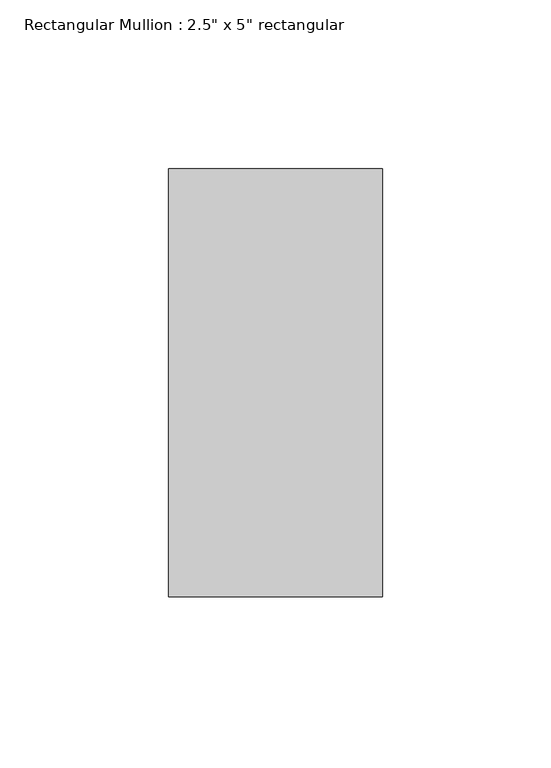
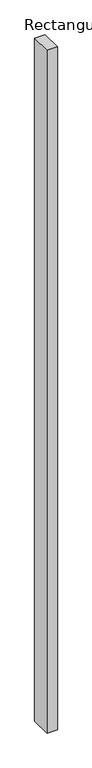
"""IFC4 building model written with IfcOpenShell, lengths in millimetres: member geometry."""

from ifc_helpers import new_model, si_unit, frame, origin, place, context, project, spatial, polyline, outline, extrude, source, transform, mapped, element, save


def member_4a27761c(model_context):
    return source(origin(), model_context, "Body", "SweptSolid", [
        extrude(outline(polyline([(0.0, 63.5), (0.0, -63.5), (-63.5, -63.5), (-63.5, 63.5), (0.0, 63.5)])), frame((0.0, 0.0, -4364.320945), z_axis=(0.0, 0.0, 1.0), x_axis=(1.0, 0.0, 0.0)), (0.0, 0.0, 1.0), 4364.320945),
    ])


if __name__ == "__main__":
    model = new_model("IFC4")
    model_context = context("Model", 3, world=origin())
    ifc_project = project(units=[si_unit("LENGTHUNIT", "METRE", prefix="MILLI")], contexts=[model_context])
    site = spatial("IfcSite", under=ifc_project)
    building = spatial("IfcBuilding", under=site)
    placement = place(None, origin())
    member_shape = member_4a27761c(model_context)
    element("IfcMember", 1, ObjectType="Rectangular Mullion : 2.5\" x 5\" rectangular", at=placement, inside=building, context=model_context, shape_type="MappedRepresentation", body=[
        mapped(member_shape, transform((0.0, 0.0, 0.0), x_axis=(1.0, 0.0, 0.0), y_axis=(0.0, 1.0, 0.0), z_axis=(0.0, 0.0, 1.0))),
    ])
    save(model, "model.ifc")

# Revit data of these elements
# Type "Rectangular Mullion : 2.5\" x 5\" rectangular"
#   built-in parameter 1007304 = 0.416667 (stored number, unit not read)
#   built-in parameter 1007301 = 0.104167 (stored number, unit not read)
#   built-in parameter 1007300 = 0.104167 (stored number, unit not read)
# Element 1 (IfcMember, "Rectangular Mullion : 2.5\" x 5\" rectangular")
#   Materials on its faces: "Aluminum"
# Materials
#   "Aluminum": class "Metal", colour RGB 247 247 247, transparency 0, Description = "Aluminum 6061", Cost = 0
